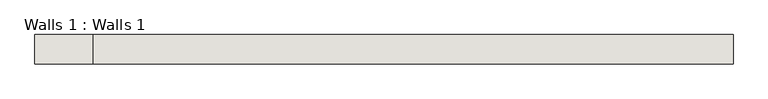
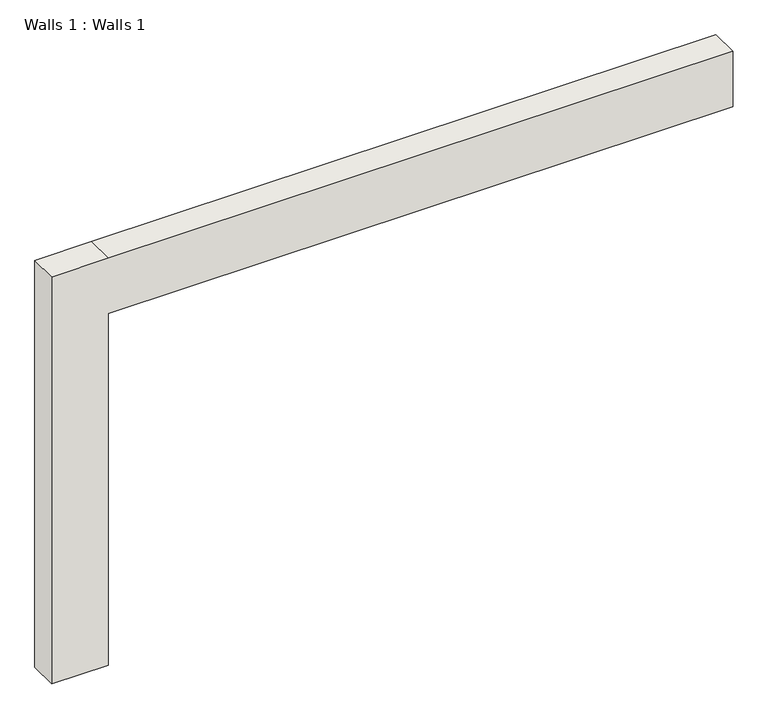
"""IFC4 building model written with IfcOpenShell, lengths in millimetres: wall geometry, Walls 1 : Walls 1."""

from ifc_helpers import new_model, si_unit, frame, origin, place, context, project, spatial, polyline, outline, extrude, source, transform, mapped, element, save


def walls_1_walls_1_592a891f(model_context):
    return source(origin(), model_context, "Body", "SweptSolid", [
        extrude(outline(polyline([(0.0, -7474.5150201), (6587.697392, -7474.5150201), (6587.697392, 3589.3688099), (7620.0, 3589.3688099), (7620.0, -7474.5150201), (7620.0, -8475.6311901), (0.0, -8475.6311901), (0.0, -7474.5150201)])), frame((0.0, -4553.7470657, 0.0), z_axis=(0.0, 1.0, 0.0), x_axis=(0.0, 0.0, 1.0)), (0.0, 0.0, 1.0), 511.2331145),
    ])


if __name__ == "__main__":
    model = new_model("IFC4")
    model_context = context("Model", 3, world=origin())
    ifc_project = project(units=[si_unit("LENGTHUNIT", "METRE", prefix="MILLI")], contexts=[model_context])
    site = spatial("IfcSite", under=ifc_project)
    building = spatial("IfcBuilding", under=site)
    placement = place(None, origin())
    walls_1_walls_1_shape = walls_1_walls_1_592a891f(model_context)
    element("IfcWall", 1, ObjectType="Walls 1 : Walls 1", at=placement, inside=building, context=model_context, shape_type="MappedRepresentation", body=[
        mapped(walls_1_walls_1_shape, transform((0.0, 0.0, 0.0), x_axis=(1.0, 0.0, 0.0), y_axis=(0.0, 1.0, 0.0), z_axis=(0.0, 0.0, 1.0))),
    ])
    save(model, "model.ifc")

# Revit data of these elements
# Element 1 (IfcWall, "Walls 1 : Walls 1")
#   Materials on its faces: "Default Wall"
# Materials
#   "Default Wall": colour RGB 128 128 128, transparency 0
